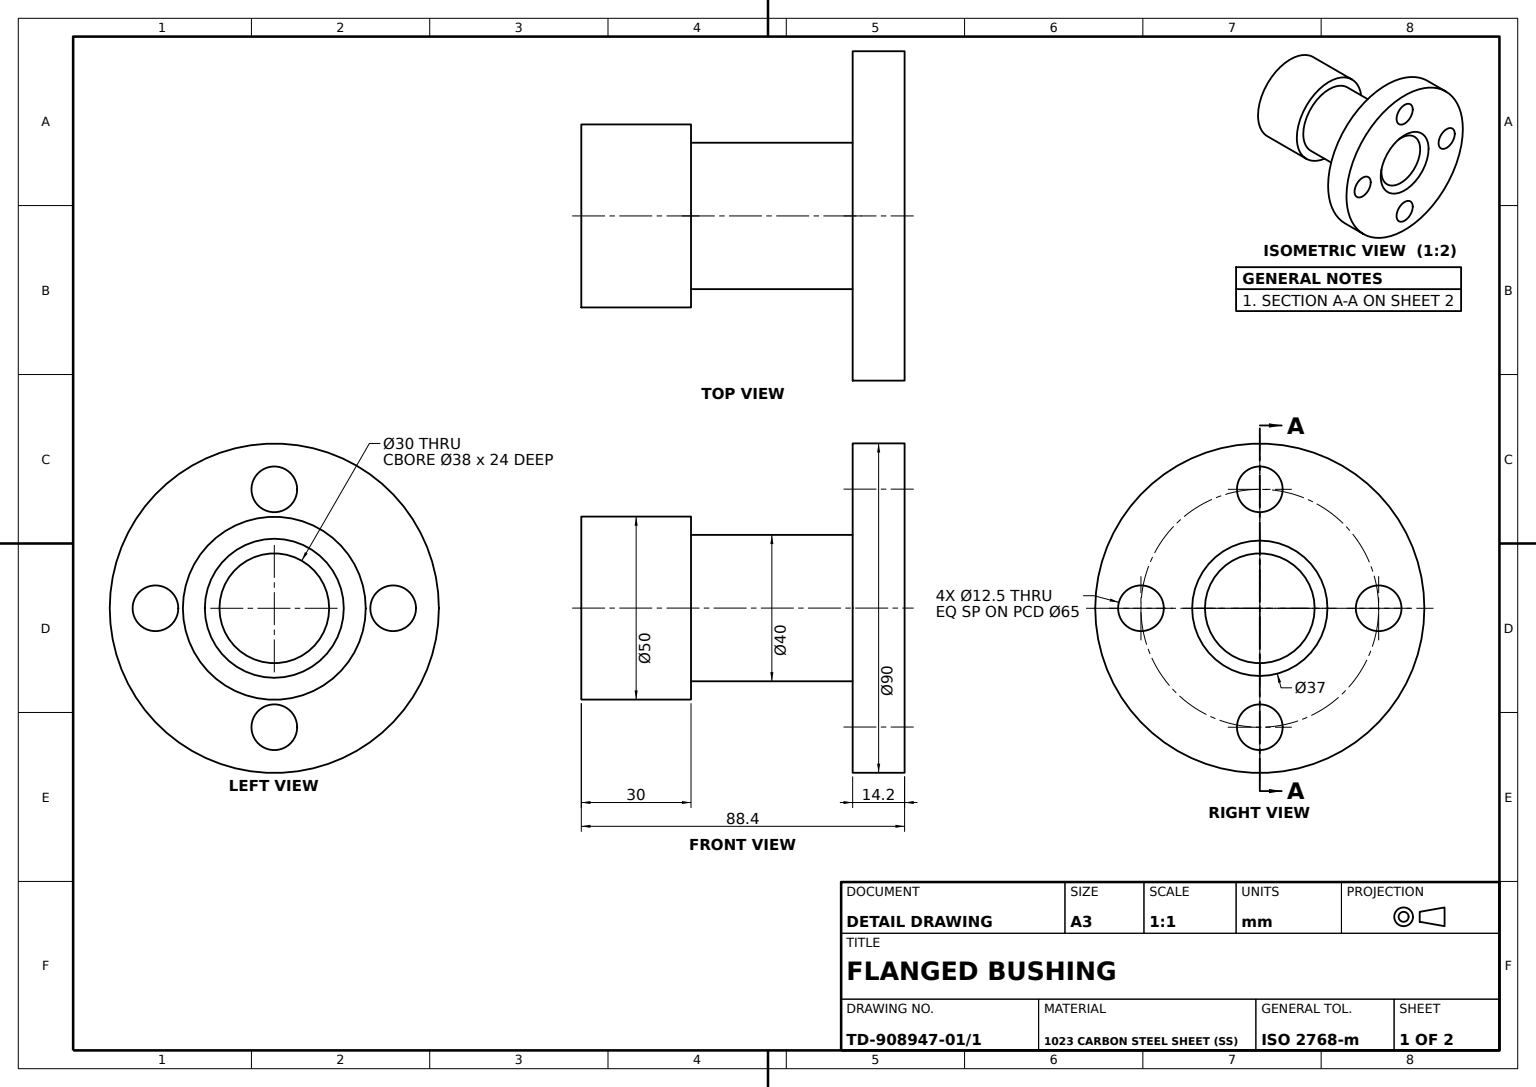
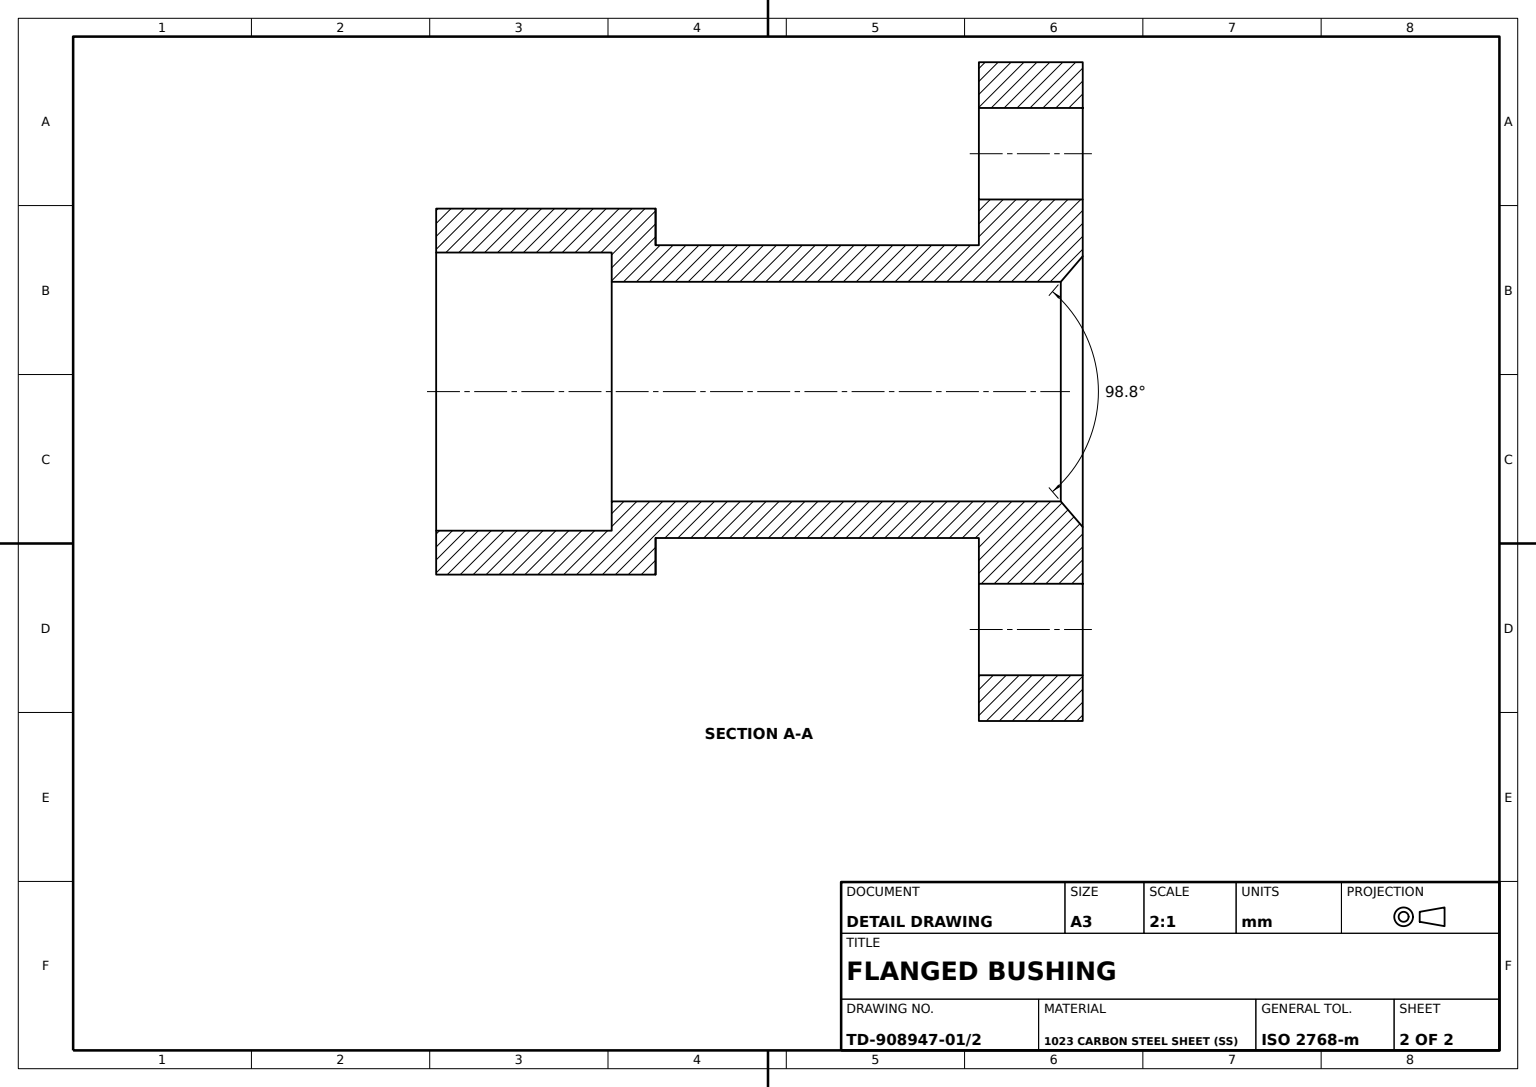
from build123d import *

# Parameters (mm, degrees)
FLANGE_SKETCH_R             = 45
FLANGE_SKETCH_R_2           = 15
FLANGE_90_DEPTH             = 14.2
HUB_SKETCH_R                = 20
HUB_SKETCH_R_2              = 15
HUB_40_DEPTH                = 44.2
COLLAR_SKETCH_R             = 25
COLLAR_SKETCH_R_2           = 15
COLLAR_50_DEPTH             = 6
END_SLEEVE_SKETCH_R         = 25
END_SLEEVE_SKETCH_R_2       = 19
END_SLEEVE_50_BORE_38_DEPTH = 24
FLANGE_EDGE_CHAMFER_SIZE    = 3
FLANGE_EDGE_CHAMFER_SIZE2   = 3.5
BOLT_HOLES_SET_A_SKETCH_R   = 6.25
BOLT_HOLES_SET_A_DEPTH      = 24
BOLT_HOLES_SET_B_SKETCH_R   = 6.25
BOLT_HOLES_SET_B_DEPTH      = 24


with BuildPart() as part:
    # Flange Sketch → Flange Ø90 (new body)
    with BuildSketch(Plane.XY):
        Circle(FLANGE_SKETCH_R)
        Circle(FLANGE_SKETCH_R_2, mode=Mode.SUBTRACT)
    extrude(amount=FLANGE_90_DEPTH)

    # Hub Sketch → Hub Ø40 (add)
    with BuildSketch(Plane.XY.offset(14.2)):
        Circle(HUB_SKETCH_R)
        Circle(HUB_SKETCH_R_2, mode=Mode.SUBTRACT)
    extrude(amount=HUB_40_DEPTH)

    # Collar Sketch → Collar Ø50 (add)
    with BuildSketch(Plane.XY.offset(58.4)):
        Circle(COLLAR_SKETCH_R)
        Circle(COLLAR_SKETCH_R_2, mode=Mode.SUBTRACT)
    extrude(amount=COLLAR_50_DEPTH)

    # End Sleeve Sketch → End Sleeve Ø50 Bore Ø38 (add)
    with BuildSketch(Plane.XY.offset(64.4)):
        Circle(END_SLEEVE_SKETCH_R)
        Circle(END_SLEEVE_SKETCH_R_2, mode=Mode.SUBTRACT)
    extrude(amount=END_SLEEVE_50_BORE_38_DEPTH)

    # Flange Edge Chamfer
    flange_edge_chamfer_edges = [part.edges().sort_by_distance(p)[0] for p in [
        (-15, 0, 0),
    ]]
    flange_edge_chamfer_side = [part.faces().sort_by_distance(p)[0] for p in [
        (-15, 0, 32.2),
    ]]
    chamfer(flange_edge_chamfer_edges, length=FLANGE_EDGE_CHAMFER_SIZE, length2=FLANGE_EDGE_CHAMFER_SIZE2, reference=flange_edge_chamfer_side[0])

    # Bolt Holes Set A Sketch → Bolt Holes Set A (cut)
    with BuildSketch(Plane.XY):
        with Locations((0, 32.5)):
            Circle(BOLT_HOLES_SET_A_SKETCH_R)
        with Locations((0, -32.5)):
            Circle(BOLT_HOLES_SET_A_SKETCH_R)
    extrude(amount=BOLT_HOLES_SET_A_DEPTH, mode=Mode.SUBTRACT)

    # Bolt Holes Set B Sketch → Bolt Holes Set B (cut)
    with BuildSketch(Plane.XY):
        with Locations((-32.5, 0)):
            Circle(BOLT_HOLES_SET_B_SKETCH_R)
        with Locations((32.5, 0)):
            Circle(BOLT_HOLES_SET_B_SKETCH_R)
    extrude(amount=BOLT_HOLES_SET_B_DEPTH, mode=Mode.SUBTRACT)


solid = part.part
